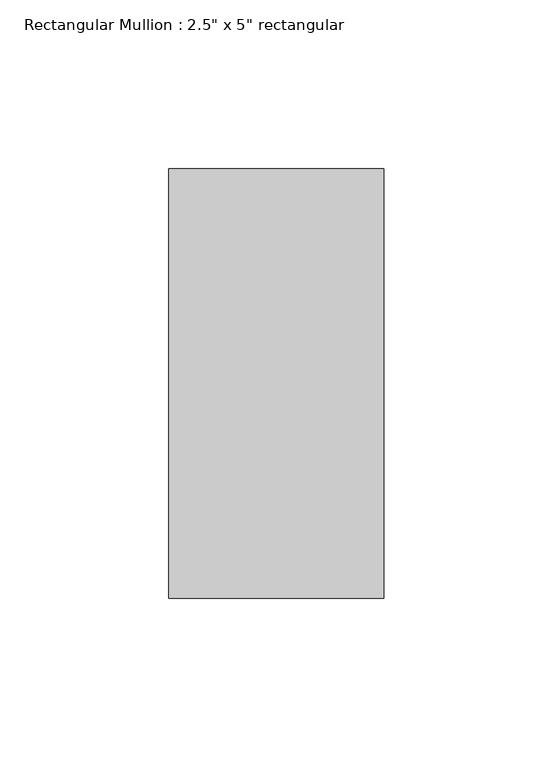
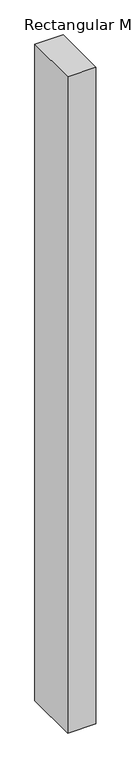
"""IFC4 building model written with IfcOpenShell, lengths in millimetres: member geometry."""

from ifc_helpers import new_model, si_unit, frame, origin, place, context, project, spatial, polyline, outline, extrude, source, transform, mapped, element, save


def member_607f7529(model_context):
    return source(origin(), model_context, "Body", "SweptSolid", [
        extrude(outline(polyline([(31.75, 63.5), (31.75, -63.5), (-31.75, -63.5), (-31.75, 63.5), (31.75, 63.5)])), frame((0.0, 0.0, -1557.4533749), z_axis=(0.0, 0.0, 1.0), x_axis=(1.0, 0.0, 0.0)), (0.0, 0.0, 1.0), 1557.4533749),
    ])


if __name__ == "__main__":
    model = new_model("IFC4")
    model_context = context("Model", 3, world=origin())
    ifc_project = project(units=[si_unit("LENGTHUNIT", "METRE", prefix="MILLI")], contexts=[model_context])
    site = spatial("IfcSite", under=ifc_project)
    building = spatial("IfcBuilding", under=site)
    placement = place(None, origin())
    member_shape = member_607f7529(model_context)
    element("IfcMember", 1, ObjectType="Rectangular Mullion : 2.5\" x 5\" rectangular", at=placement, inside=building, context=model_context, shape_type="MappedRepresentation", body=[
        mapped(member_shape, transform((0.0, 0.0, 0.0), x_axis=(1.0, 0.0, 0.0), y_axis=(0.0, 1.0, 0.0), z_axis=(0.0, 0.0, 1.0))),
    ])
    save(model, "model.ifc")

# Revit data of these elements
# Type "Rectangular Mullion : 2.5\" x 5\" rectangular"
#   built-in parameter 1007304 = 0.416667 (stored number, unit not read)
#   built-in parameter 1007301 = 0.104167 (stored number, unit not read)
#   built-in parameter 1007300 = 0.104167 (stored number, unit not read)
# Element 1 (IfcMember, "Rectangular Mullion : 2.5\" x 5\" rectangular")
#   Materials on its faces: "Aluminum"
# Materials
#   "Aluminum": class "Metal", colour RGB 247 247 247, transparency 0, Description = "Aluminum 6061", Cost = 0
